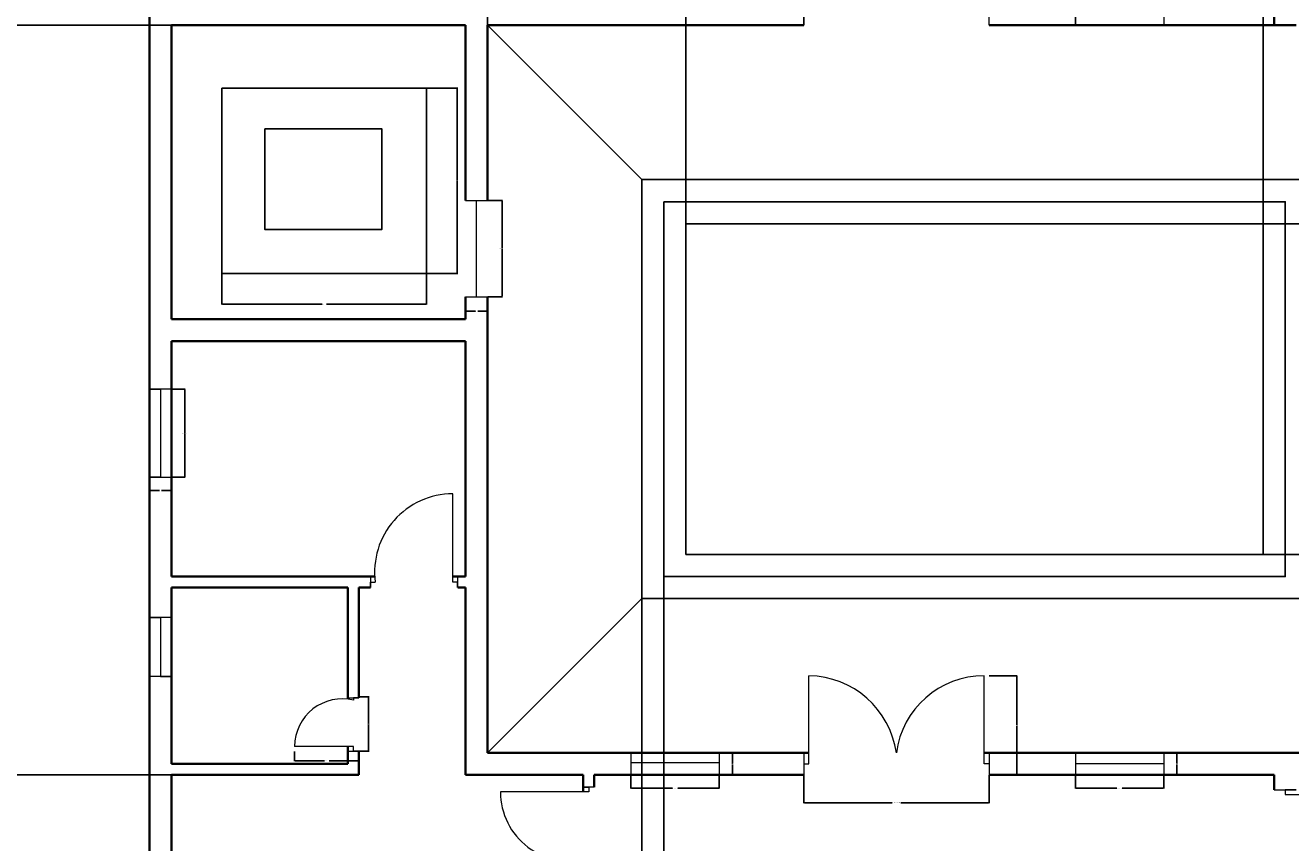
# Model space of a CAD drawing. Units: inches. Extents: x 2185 to 4426, y 1138 to 3073.
# Tile 9 of 14: x 3160 to 3677, y 1501 to 1834. Entities that reach past the tile are written whole.
import ezdxf

# ---------------------------------------------------------------- set-up
doc = ezdxf.new("R2010")
doc.units = ezdxf.units.IN
for name, color, linetype, lineweight in [('A-ANNO-DIMS', 2, 'Continuous', 18), ('A-DOOR', 3, 'Continuous', 18), ('A-FLOR-EDGE', 7, 'Continuous', 25), ('A-GLAZ', 4, 'Continuous', 18), ('A-SITE-WELL', 7, 'Continuous', 25), ('A-WALL', 7, 'Continuous', 35)]:
    doc.layers.add(name, color=color, linetype=linetype, lineweight=lineweight)
doc.styles.get("Standard").update_dxf_attribs({"font": 'arial.ttf'})
doc.dimstyles.get("Standard").update_dxf_attribs({"dimtxt": 0.18, "dimasz": 0.18, "dimexe": 0.18, "dimexo": 0.0625, "dimgap": 0.09, "dimtad": 0, "dimtih": 1, "dimtoh": 1, "dimdec": 4, "dimzin": 0, "dimdsep": 46, "dimtxsty": 'Standard', "dimcen": 0.09, "dimadec": 0, "dimazin": 0, "dimtfac": 1, "dimtdec": 4, "dimtofl": 0, "dimtmove": 0, "dimatfit": 3, "dimfxl": 1, "dimtolj": 1, "dimtzin": 0, "dimarcsym": 0})

# ---------------------------------------------------------------- blocks, each defined once
blk = doc.blocks.new('DOOR-SGL-24-BATH-W')
for p, q in [((21.75, 21.83), (26.25, 21.83)), ((26.25, 21.83), (24, 21.83)), ((24, 21.83), (24, 20.83)), ((24, 2), (0, 2)), ((24, 0), (24, 2)), ((21.75, 0), (26.25, 0)), ((26.25, 0), (24, 0))]:
    blk.add_line(p, q)
blk.add_arc((19.38, 2), 19.38, 76.226, 180)
blk = doc.blocks.new('DOOR-SGL-36-READING')
for p, q in [((33.62, 2.25), (33.62, 38.25)), ((0, 4.5), (0, 0)), ((0, 0), (0, 2.25)), ((0, 2.25), (2, 2.25)), ((35.62, 2.25), (33.62, 2.25)), ((35.62, 4.5), (35.62, 0)), ((35.62, 0), (35.62, 2.25))]:
    blk.add_line(p, q)
blk.add_arc((33.62, 6.36), 31.89, 90, 187.4032)
blk = doc.blocks.new('DOOR-PAIR-36-DINING')
for p, q in [((2, 4.5), (2, 40.5)), ((73.51, 4.5), (73.51, 40.5)), ((0, 9), (0, 0)), ((75.51, 0), (75.51, 9)), ((75.51, 9), (75.51, 4.5)), ((0, 0), (0, 4.5)), ((0, 4.5), (2, 4.5)), ((75.51, 4.5), (73.51, 4.5))]:
    blk.add_line(p, q)
for centre, radius, start, end in [((2, 3.7), 36.8, 8.2761, 90), ((74.14, 4.5), 36.01, 90.9934, 172.8203)]:
    blk.add_arc(centre, radius, start, end)
blk = doc.blocks.new('DOOR-SGL-36-BED-SW')
for p, q in [((38.25, 31.13), (33.75, 31.13)), ((33.75, 31.13), (36, 31.13)), ((36, 31.13), (36, 29.13)), ((36, 29.13), (0, 29.13)), ((36, 0), (36, 2)), ((33.75, 0), (38.25, 0)), ((38.25, 0), (36, 0))]:
    blk.add_line(p, q)
blk.add_arc((28.22, 29.13), 28.22, 180, 285.9925)
blk = doc.blocks.new('DOOR-PAIR-36-VERANDA')
for p, q in [((2, 4.5), (2, 40.5)), ((73.51, 4.5), (73.51, 40.5)), ((0, 9), (0, 0)), ((75.51, 9), (75.51, 0)), ((0, 4.5), (2, 4.5)), ((75.51, 4.5), (73.51, 4.5))]:
    blk.add_line(p, q)
for centre, radius, start, end in [((1.42, 3.87), 36.64, 8.0545, 89.0928), ((73.51, 4.39), 36.11, 90, 172.6635)]:
    blk.add_arc(centre, radius, start, end)
blk = doc.blocks.new('DOOR-SGL-36-BED-S')
for p, q in [((0, 31.73), (9, 31.73)), ((9, 31.73), (4.5, 31.73)), ((4.5, 31.73), (4.5, 31.73)), ((4.5, 31.73), (4.5, 29.73)), ((4.5, 29.73), (40.5, 29.73)), ((0, 0), (9, 0)), ((4.5, 0), (4.5, 2)), ((9, 0), (4.5, 0))]:
    blk.add_line(p, q)
blk.add_arc((11.82, 29.73), 28.68, 255.2109, 0)
blk = doc.blocks.new('WIN-PLAN-24IN-02')
for p, q in [((9, 24), (0, 24)), ((0, 24), (4.5, 24)), ((4.5, 24), (4.5, 0)), ((9, 0), (0, 0)), ((0, 0), (0, 0)), ((4.5, 0), (9, 0))]:
    blk.add_line(p, q)
blk = doc.blocks.new('WIN-PLAN-36IN-01')
for p, q in [((0, 9), (0, 0)), ((36, 4.5), (36, 9)), ((36, 9), (36, 0)), ((0, 0), (0, 4.5)), ((0, 4.5), (0, 4.5)), ((0, 4.5), (36, 4.5))]:
    blk.add_line(p, q)
blk = doc.blocks.new('WIN-PLAN-36IN-03')
for p, q in [((9, 36), (0, 36)), ((0, 36), (0, 36)), ((0, 36), (4.5, 36)), ((4.5, 36), (4.5, 0)), ((4.5, 0), (0, 0)), ((0, 0), (9, 0)), ((9, 0), (9, 0))]:
    blk.add_line(p, q)
blk = doc.blocks.new('WIN-PLAN-36IN-06')
for p, q in [((0, 9), (0, 0)), ((36, 9), (36, 0)), ((0, 5.12), (36, 5.12)), ((36, 5.12), (36, 5.12))]:
    blk.add_line(p, q)
blk = doc.blocks.new('WIN-PLAN-36IN-07')
for p, q in [((0, 9), (0, 0)), ((36, 9), (36, 0)), ((36, 4.5), (0, 4.5))]:
    blk.add_line(p, q)
blk = doc.blocks.new('WIN-PLAN-39IN')
for p, q in [((0, 39.26), (9, 39.26)), ((4.5, 0), (4.5, 39.26)), ((0, 0), (9, 0))]:
    blk.add_line(p, q)
blk = doc.blocks.new('WELL-PLAN')
for points in [[(0, 75.64), (83.5, 75.64), (83.5, 0), (0, 0)], [(17.44, 59), (65.29, 59), (65.29, 18), (17.44, 18)]]:
    blk.add_lwpolyline(points, close=True)
blk = doc.blocks.new('*D72')
at = {"layer": 'A-ANNO-DIMS', "color": 0, "lineweight": -2, "transparency": 16777216}
for p, q in [((3270.1, 1537.99), (3270.1, 1533.94)), ((3270.28, 1534.12), (3282.29, 1534.12)), ((3296.17, 1534.12), (3284.16, 1534.12)), ((3296.35, 1537.99), (3296.35, 1533.94))]:
    blk.add_line(p, q, dxfattribs=at)
at = {"layer": 'A-ANNO-DIMS', "color": 0, "transparency": 16777216}
for points in [[(3270.28, 1534.15), (3270.28, 1534.09), (3270.1, 1534.12)], [(3296.17, 1534.15), (3296.17, 1534.09), (3296.35, 1534.12)]]:
    blk.add_solid(points, dxfattribs=at)
at = {"layer": 'Defpoints', "color": 0, "transparency": 16777216}
for p in [(3270.1, 1538.05), (3296.35, 1538.05), (3296.35, 1534.12)]:
    blk.add_point(p, dxfattribs=at)
at = {"layer": 'A-ANNO-DIMS', "color": 0, "transparency": 16777216, "insert": (3283.22, 1534.12), "char_height": 0.18, "attachment_point": 5}
blk.add_mtext('\\A1;DOOR 26 TYP.', dxfattribs=at)
blk = doc.blocks.new('*D73')
at = {"layer": 'A-ANNO-DIMS', "color": 0, "lineweight": -2, "transparency": 16777216}
for p, q in [((3296.41, 1560.3), (3300.47, 1560.3)), ((3300.29, 1560.12), (3300.29, 1549.36)), ((3300.29, 1538.23), (3300.29, 1549)), ((3296.41, 1538.05), (3300.47, 1538.05))]:
    blk.add_line(p, q, dxfattribs=at)
at = {"layer": 'A-ANNO-DIMS', "color": 0, "transparency": 16777216}
for points in [[(3300.26, 1560.12), (3300.32, 1560.12), (3300.29, 1560.3)], [(3300.26, 1538.23), (3300.32, 1538.23), (3300.29, 1538.05)]]:
    blk.add_solid(points, dxfattribs=at)
at = {"layer": 'Defpoints', "color": 0, "transparency": 16777216}
for p in [(3296.35, 1560.3), (3300.29, 1560.3), (3296.35, 1538.05)]:
    blk.add_point(p, dxfattribs=at)
at = {"layer": 'A-ANNO-DIMS', "color": 0, "transparency": 16777216, "insert": (3300.29, 1549.18), "char_height": 0.18, "attachment_point": 5}
blk.add_mtext('\\A1;22 TYP.', dxfattribs=at)
blk = doc.blocks.new('*D86')
at = {"layer": 'A-ANNO-DIMS', "color": 0, "lineweight": -2, "transparency": 16777216}
for p, q in [((3477.97, 1528.31), (3477.97, 1516.87)), ((3553.49, 1528.31), (3553.49, 1516.87)), ((3478.15, 1517.05), (3513.97, 1517.05)), ((3553.31, 1517.05), (3517.49, 1517.05))]:
    blk.add_line(p, q, dxfattribs=at)
at = {"layer": 'A-ANNO-DIMS', "color": 0, "transparency": 16777216}
for points in [[(3478.15, 1517.08), (3478.15, 1517.02), (3477.97, 1517.05)], [(3553.31, 1517.08), (3553.31, 1517.02), (3553.49, 1517.05)]]:
    blk.add_solid(points, dxfattribs=at)
at = {"layer": 'Defpoints', "color": 0, "transparency": 16777216}
for p in [(3477.97, 1528.38), (3553.49, 1528.38), (3553.49, 1517.05)]:
    blk.add_point(p, dxfattribs=at)
at = {"layer": 'A-ANNO-DIMS', "color": 0, "transparency": 16777216, "insert": (3515.73, 1517.05), "char_height": 0.18, "attachment_point": 5}
blk.add_mtext('\\A1;VERANDAH DOORS 76 TYP.', dxfattribs=at)
blk = doc.blocks.new('*D87')
at = {"layer": 'A-ANNO-DIMS', "color": 0, "lineweight": -2, "transparency": 16777216}
for p, q in [((3553.55, 1568.88), (3564.99, 1568.88)), ((3564.81, 1568.7), (3564.81, 1548.81)), ((3564.81, 1528.56), (3564.81, 1548.45)), ((3553.55, 1528.38), (3564.99, 1528.38))]:
    blk.add_line(p, q, dxfattribs=at)
at = {"layer": 'A-ANNO-DIMS', "color": 0, "transparency": 16777216}
for points in [[(3564.78, 1568.7), (3564.84, 1568.7), (3564.81, 1568.88)], [(3564.78, 1528.56), (3564.84, 1528.56), (3564.81, 1528.38)]]:
    blk.add_solid(points, dxfattribs=at)
at = {"layer": 'Defpoints', "color": 0, "transparency": 16777216}
for p in [(3553.49, 1568.88), (3564.81, 1568.88), (3553.49, 1528.38)]:
    blk.add_point(p, dxfattribs=at)
at = {"layer": 'A-ANNO-DIMS', "color": 0, "transparency": 16777216, "insert": (3564.81, 1548.63), "char_height": 0.18, "attachment_point": 5}
blk.add_mtext('\\A1;41 TYP.', dxfattribs=at)
blk = doc.blocks.new('*D96')
at = {"layer": 'A-ANNO-DIMS', "color": 0, "lineweight": -2, "transparency": 16777216}
for p, q in [((3219.91, 1685.88), (3225.43, 1685.88)), ((3225.25, 1685.7), (3225.25, 1668.07)), ((3225.25, 1650.06), (3225.25, 1667.7)), ((3219.91, 1649.88), (3225.43, 1649.88))]:
    blk.add_line(p, q, dxfattribs=at)
at = {"layer": 'A-ANNO-DIMS', "color": 0, "transparency": 16777216}
for points in [[(3225.22, 1685.7), (3225.28, 1685.7), (3225.25, 1685.88)], [(3225.22, 1650.06), (3225.28, 1650.06), (3225.25, 1649.88)]]:
    blk.add_solid(points, dxfattribs=at)
at = {"layer": 'Defpoints', "color": 0, "transparency": 16777216}
for p in [(3219.85, 1685.88), (3225.25, 1685.88), (3219.85, 1649.88)]:
    blk.add_point(p, dxfattribs=at)
at = {"layer": 'A-ANNO-DIMS', "color": 0, "transparency": 16777216, "insert": (3225.25, 1667.88), "char_height": 0.18, "attachment_point": 5}
blk.add_mtext('\\A1;WINDOW 36 TYP.', dxfattribs=at)
blk = doc.blocks.new('*D97')
at = {"layer": 'A-ANNO-DIMS', "color": 0, "lineweight": -2, "transparency": 16777216}
for p, q in [((3210.85, 1649.82), (3210.85, 1644.3)), ((3219.85, 1649.82), (3219.85, 1644.3)), ((3211.03, 1644.48), (3214.89, 1644.48)), ((3219.67, 1644.48), (3215.81, 1644.48))]:
    blk.add_line(p, q, dxfattribs=at)
at = {"layer": 'A-ANNO-DIMS', "color": 0, "transparency": 16777216}
for points in [[(3211.03, 1644.51), (3211.03, 1644.45), (3210.85, 1644.48)], [(3219.67, 1644.51), (3219.67, 1644.45), (3219.85, 1644.48)]]:
    blk.add_solid(points, dxfattribs=at)
at = {"layer": 'Defpoints', "color": 0, "transparency": 16777216}
for p in [(3210.85, 1649.88), (3219.85, 1649.88), (3219.85, 1644.48)]:
    blk.add_point(p, dxfattribs=at)
at = {"layer": 'A-ANNO-DIMS', "color": 0, "transparency": 16777216, "insert": (3215.35, 1644.48), "char_height": 0.18, "attachment_point": 5}
blk.add_mtext('\\A1;9 TYP.', dxfattribs=at)
blk = doc.blocks.new('*D102')
at = {"layer": 'A-ANNO-DIMS', "color": 0, "lineweight": -2, "transparency": 16777216}
for p, q in [((3407.37, 1528.31), (3407.37, 1522.8)), ((3443.37, 1528.31), (3443.37, 1522.8)), ((3407.55, 1522.98), (3424.25, 1522.98)), ((3443.19, 1522.98), (3426.49, 1522.98))]:
    blk.add_line(p, q, dxfattribs=at)
at = {"layer": 'A-ANNO-DIMS', "color": 0, "transparency": 16777216}
for points in [[(3407.55, 1523.01), (3407.55, 1522.95), (3407.37, 1522.98)], [(3443.19, 1523.01), (3443.19, 1522.95), (3443.37, 1522.98)]]:
    blk.add_solid(points, dxfattribs=at)
at = {"layer": 'Defpoints', "color": 0, "transparency": 16777216}
for p in [(3407.37, 1528.38), (3443.37, 1528.38), (3443.37, 1522.98)]:
    blk.add_point(p, dxfattribs=at)
at = {"layer": 'A-ANNO-DIMS', "color": 0, "transparency": 16777216, "insert": (3425.37, 1522.98), "char_height": 0.18, "attachment_point": 5}
blk.add_mtext('\\A1;WINDOW 36 TYP.', dxfattribs=at)
blk = doc.blocks.new('*D103')
at = {"layer": 'A-ANNO-DIMS', "color": 0, "lineweight": -2, "transparency": 16777216}
for p, q in [((3443.43, 1537.38), (3448.95, 1537.38)), ((3448.77, 1537.2), (3448.77, 1533.06)), ((3448.77, 1528.56), (3448.77, 1532.7)), ((3443.43, 1528.38), (3448.95, 1528.38))]:
    blk.add_line(p, q, dxfattribs=at)
at = {"layer": 'A-ANNO-DIMS', "color": 0, "transparency": 16777216}
for points in [[(3448.74, 1537.2), (3448.8, 1537.2), (3448.77, 1537.38)], [(3448.74, 1528.56), (3448.8, 1528.56), (3448.77, 1528.38)]]:
    blk.add_solid(points, dxfattribs=at)
at = {"layer": 'Defpoints', "color": 0, "transparency": 16777216}
for p in [(3443.37, 1537.38), (3448.77, 1537.38), (3443.37, 1528.38)]:
    blk.add_point(p, dxfattribs=at)
at = {"layer": 'A-ANNO-DIMS', "color": 0, "transparency": 16777216, "insert": (3448.77, 1532.88), "char_height": 0.18, "attachment_point": 5}
blk.add_mtext('\\A1;9 TYP.', dxfattribs=at)
blk = doc.blocks.new('*D104')
at = {"layer": 'A-ANNO-DIMS', "color": 0, "lineweight": -2, "transparency": 16777216}
for p, q in [((3588.76, 1528.31), (3588.76, 1522.8)), ((3624.76, 1528.31), (3624.76, 1522.8)), ((3588.94, 1522.98), (3605.64, 1522.98)), ((3624.58, 1522.98), (3607.88, 1522.98))]:
    blk.add_line(p, q, dxfattribs=at)
at = {"layer": 'A-ANNO-DIMS', "color": 0, "transparency": 16777216}
for points in [[(3588.94, 1523.01), (3588.94, 1522.95), (3588.76, 1522.98)], [(3624.58, 1523.01), (3624.58, 1522.95), (3624.76, 1522.98)]]:
    blk.add_solid(points, dxfattribs=at)
at = {"layer": 'Defpoints', "color": 0, "transparency": 16777216}
for p in [(3588.76, 1528.38), (3624.76, 1528.38), (3624.76, 1522.98)]:
    blk.add_point(p, dxfattribs=at)
at = {"layer": 'A-ANNO-DIMS', "color": 0, "transparency": 16777216, "insert": (3606.76, 1522.98), "char_height": 0.18, "attachment_point": 5}
blk.add_mtext('\\A1;WINDOW 36 TYP.', dxfattribs=at)
blk = doc.blocks.new('*D105')
at = {"layer": 'A-ANNO-DIMS', "color": 0, "lineweight": -2, "transparency": 16777216}
for p, q in [((3624.82, 1537.38), (3630.34, 1537.38)), ((3630.16, 1537.2), (3630.16, 1533.06)), ((3630.16, 1528.56), (3630.16, 1532.7)), ((3624.82, 1528.38), (3630.34, 1528.38))]:
    blk.add_line(p, q, dxfattribs=at)
at = {"layer": 'A-ANNO-DIMS', "color": 0, "transparency": 16777216}
for points in [[(3630.13, 1537.2), (3630.19, 1537.2), (3630.16, 1537.38)], [(3630.13, 1528.56), (3630.19, 1528.56), (3630.16, 1528.38)]]:
    blk.add_solid(points, dxfattribs=at)
at = {"layer": 'Defpoints', "color": 0, "transparency": 16777216}
for p in [(3624.76, 1537.38), (3630.16, 1537.38), (3624.76, 1528.38)]:
    blk.add_point(p, dxfattribs=at)
at = {"layer": 'A-ANNO-DIMS', "color": 0, "transparency": 16777216, "insert": (3630.16, 1532.88), "char_height": 0.18, "attachment_point": 5}
blk.add_mtext('\\A1;9 TYP.', dxfattribs=at)
blk = doc.blocks.new('*D112')
at = {"layer": 'A-ANNO-DIMS', "color": 0, "lineweight": -2, "transparency": 16777216}
for p, q in [((3348.91, 1762.84), (3354.92, 1762.84)), ((3354.74, 1762.66), (3354.74, 1743.4)), ((3354.74, 1723.77), (3354.74, 1743.03)), ((3348.91, 1723.59), (3354.92, 1723.59))]:
    blk.add_line(p, q, dxfattribs=at)
at = {"layer": 'A-ANNO-DIMS', "color": 0, "transparency": 16777216}
for points in [[(3354.71, 1762.66), (3354.77, 1762.66), (3354.74, 1762.84)], [(3354.71, 1723.77), (3354.77, 1723.77), (3354.74, 1723.59)]]:
    blk.add_solid(points, dxfattribs=at)
at = {"layer": 'Defpoints', "color": 0, "transparency": 16777216}
for p in [(3348.85, 1762.84), (3354.74, 1762.84), (3348.85, 1723.59)]:
    blk.add_point(p, dxfattribs=at)
at = {"layer": 'A-ANNO-DIMS', "color": 0, "transparency": 16777216, "insert": (3354.74, 1743.21), "char_height": 0.18, "attachment_point": 5}
blk.add_mtext('\\A1;WINDOW 39 TYP.', dxfattribs=at)
blk = doc.blocks.new('*D113')
at = {"layer": 'A-ANNO-DIMS', "color": 0, "lineweight": -2, "transparency": 16777216}
for p, q in [((3339.85, 1723.52), (3339.85, 1717.52)), ((3348.85, 1723.52), (3348.85, 1717.52)), ((3340.03, 1717.7), (3343.89, 1717.7)), ((3348.67, 1717.7), (3344.81, 1717.7))]:
    blk.add_line(p, q, dxfattribs=at)
at = {"layer": 'A-ANNO-DIMS', "color": 0, "transparency": 16777216}
for points in [[(3340.03, 1717.73), (3340.03, 1717.67), (3339.85, 1717.7)], [(3348.67, 1717.73), (3348.67, 1717.67), (3348.85, 1717.7)]]:
    blk.add_solid(points, dxfattribs=at)
at = {"layer": 'Defpoints', "color": 0, "transparency": 16777216}
for p in [(3339.85, 1723.59), (3348.85, 1723.59), (3348.85, 1717.7)]:
    blk.add_point(p, dxfattribs=at)
at = {"layer": 'A-ANNO-DIMS', "color": 0, "transparency": 16777216, "insert": (3344.35, 1717.7), "char_height": 0.18, "attachment_point": 5}
blk.add_mtext('\\A1;9 TYP.', dxfattribs=at)
blk = doc.blocks.new('*D118')
at = {"layer": 'A-ANNO-DIMS', "color": 0, "lineweight": -2, "transparency": 16777216}
for p, q in [((3240.45, 1733), (3240.45, 1720.36)), ((3323.95, 1733), (3323.95, 1720.36)), ((3240.63, 1720.54), (3281.29, 1720.54)), ((3323.77, 1720.54), (3283.11, 1720.54))]:
    blk.add_line(p, q, dxfattribs=at)
at = {"layer": 'A-ANNO-DIMS', "color": 0, "transparency": 16777216}
for points in [[(3240.63, 1720.57), (3240.63, 1720.51), (3240.45, 1720.54)], [(3323.77, 1720.57), (3323.77, 1720.51), (3323.95, 1720.54)]]:
    blk.add_solid(points, dxfattribs=at)
at = {"layer": 'Defpoints', "color": 0, "transparency": 16777216}
for p in [(3240.45, 1733.06), (3323.95, 1733.06), (3323.95, 1720.54)]:
    blk.add_point(p, dxfattribs=at)
at = {"layer": 'A-ANNO-DIMS', "color": 0, "transparency": 16777216, "insert": (3282.2, 1720.54), "char_height": 0.18, "attachment_point": 5}
blk.add_mtext('\\A1;WELL 84 TYP.', dxfattribs=at)
blk = doc.blocks.new('*D119')
at = {"layer": 'A-ANNO-DIMS', "color": 0, "lineweight": -2, "transparency": 16777216}
for p, q in [((3324.01, 1808.7), (3336.66, 1808.7)), ((3336.48, 1808.52), (3336.48, 1771.06)), ((3336.48, 1733.24), (3336.48, 1770.7)), ((3324.01, 1733.06), (3336.66, 1733.06))]:
    blk.add_line(p, q, dxfattribs=at)
at = {"layer": 'A-ANNO-DIMS', "color": 0, "transparency": 16777216}
for points in [[(3336.45, 1808.52), (3336.51, 1808.52), (3336.48, 1808.7)], [(3336.45, 1733.24), (3336.51, 1733.24), (3336.48, 1733.06)]]:
    blk.add_solid(points, dxfattribs=at)
at = {"layer": 'Defpoints', "color": 0, "transparency": 16777216}
for p in [(3323.95, 1808.7), (3336.48, 1808.7), (3323.95, 1733.06)]:
    blk.add_point(p, dxfattribs=at)
at = {"layer": 'A-ANNO-DIMS', "color": 0, "transparency": 16777216, "insert": (3336.48, 1770.88), "char_height": 0.18, "attachment_point": 5}
blk.add_mtext('\\A1;76 TYP.', dxfattribs=at)
blk = doc.blocks.new('*D150')
at = {"layer": 'A-ANNO-DIMS', "color": 0, "lineweight": -2, "transparency": 16777216}
for p, q in [((3219.79, 1528.38), (3101.64, 1528.38)), ((3101.82, 1528.2), (3101.82, 1428.06)), ((3101.82, 1327.56), (3101.82, 1427.7)), ((3210.79, 1327.38), (3101.64, 1327.38))]:
    blk.add_line(p, q, dxfattribs=at)
at = {"layer": 'A-ANNO-DIMS', "color": 0, "transparency": 16777216}
for points in [[(3101.79, 1528.2), (3101.85, 1528.2), (3101.82, 1528.38)], [(3101.79, 1327.56), (3101.85, 1327.56), (3101.82, 1327.38)]]:
    blk.add_solid(points, dxfattribs=at)
at = {"layer": 'Defpoints', "color": 0, "transparency": 16777216}
for p in [(3101.82, 1528.38), (3219.85, 1528.38), (3210.85, 1327.38)]:
    blk.add_point(p, dxfattribs=at)
at = {"layer": 'A-ANNO-DIMS', "color": 0, "transparency": 16777216, "insert": (3101.82, 1427.88), "char_height": 0.18, "attachment_point": 5}
blk.add_mtext('\\A1;201', dxfattribs=at)
blk = doc.blocks.new('*D151')
at = {"layer": 'A-ANNO-DIMS', "color": 0, "lineweight": -2, "transparency": 16777216}
for p, q in [((3219.79, 1834.38), (3101.64, 1834.38)), ((3101.82, 1834.2), (3101.82, 1681.56)), ((3101.82, 1528.56), (3101.82, 1681.19)), ((3219.79, 1528.38), (3101.64, 1528.38))]:
    blk.add_line(p, q, dxfattribs=at)
at = {"layer": 'A-ANNO-DIMS', "color": 0, "transparency": 16777216}
for points in [[(3101.79, 1834.2), (3101.85, 1834.2), (3101.82, 1834.38)], [(3101.79, 1528.56), (3101.85, 1528.56), (3101.82, 1528.38)]]:
    blk.add_solid(points, dxfattribs=at)
at = {"layer": 'Defpoints', "color": 0, "transparency": 16777216}
for p in [(3101.82, 1834.38), (3219.85, 1834.38), (3219.85, 1528.38)]:
    blk.add_point(p, dxfattribs=at)
at = {"layer": 'A-ANNO-DIMS', "color": 0, "transparency": 16777216, "insert": (3101.82, 1681.38), "char_height": 0.18, "attachment_point": 5}
blk.add_mtext('\\A1;306', dxfattribs=at)
blk = doc.blocks.new('*D152')
at = {"layer": 'A-ANNO-DIMS', "color": 0, "lineweight": -2, "transparency": 16777216}
for p, q in [((3155.01, 1880.56), (3101.64, 1880.56)), ((3101.82, 1880.38), (3101.82, 1857.65)), ((3101.82, 1834.56), (3101.82, 1857.29)), ((3219.79, 1834.38), (3101.64, 1834.38))]:
    blk.add_line(p, q, dxfattribs=at)
at = {"layer": 'A-ANNO-DIMS', "color": 0, "transparency": 16777216}
for points in [[(3101.79, 1880.38), (3101.85, 1880.38), (3101.82, 1880.56)], [(3101.79, 1834.56), (3101.85, 1834.56), (3101.82, 1834.38)]]:
    blk.add_solid(points, dxfattribs=at)
at = {"layer": 'Defpoints', "color": 0, "transparency": 16777216}
for p in [(3101.82, 1880.56), (3155.07, 1880.56), (3219.85, 1834.38)]:
    blk.add_point(p, dxfattribs=at)
at = {"layer": 'A-ANNO-DIMS', "color": 0, "transparency": 16777216, "insert": (3101.82, 1857.47), "char_height": 0.18, "attachment_point": 5}
blk.add_mtext('\\A1;46.19', dxfattribs=at)
blk = doc.blocks.new('*D155')
at = {"layer": 'A-ANNO-DIMS', "color": 0, "lineweight": -2, "transparency": 16777216}
for p, q in [((3348.85, 1834.44), (3348.85, 2379.81)), ((3349.03, 2379.63), (3388.93, 2379.63)), ((3429.63, 2379.63), (3389.72, 2379.63)), ((3429.81, 1753.44), (3429.81, 2379.81))]:
    blk.add_line(p, q, dxfattribs=at)
at = {"layer": 'A-ANNO-DIMS', "color": 0, "transparency": 16777216}
for points in [[(3349.03, 2379.66), (3349.03, 2379.6), (3348.85, 2379.63)], [(3429.63, 2379.66), (3429.63, 2379.6), (3429.81, 2379.63)]]:
    blk.add_solid(points, dxfattribs=at)
at = {"layer": 'Defpoints', "color": 0, "transparency": 16777216}
for p in [(3429.81, 2379.63), (3348.85, 1834.38), (3429.81, 1753.38)]:
    blk.add_point(p, dxfattribs=at)
at = {"layer": 'A-ANNO-DIMS', "color": 0, "transparency": 16777216, "insert": (3389.33, 2379.63), "char_height": 0.18, "attachment_point": 5}
blk.add_mtext('\\A1;80.96', dxfattribs=at)
blk = doc.blocks.new('*D156')
at = {"layer": 'A-ANNO-DIMS', "color": 0, "lineweight": -2, "transparency": 16777216}
for p, q in [((3429.81, 1753.44), (3429.81, 2379.81)), ((3429.99, 2379.63), (3547.11, 2379.63)), ((3665.17, 2379.63), (3548.04, 2379.63)), ((3665.35, 1753.44), (3665.35, 2379.81))]:
    blk.add_line(p, q, dxfattribs=at)
at = {"layer": 'A-ANNO-DIMS', "color": 0, "transparency": 16777216}
for points in [[(3429.99, 2379.66), (3429.99, 2379.6), (3429.81, 2379.63)], [(3665.17, 2379.66), (3665.17, 2379.6), (3665.35, 2379.63)]]:
    blk.add_solid(points, dxfattribs=at)
at = {"layer": 'Defpoints', "color": 0, "transparency": 16777216}
for p in [(3665.35, 2379.63), (3429.81, 1753.38), (3665.35, 1753.38)]:
    blk.add_point(p, dxfattribs=at)
at = {"layer": 'A-ANNO-DIMS', "color": 0, "transparency": 16777216, "insert": (3547.58, 2379.63), "char_height": 0.18, "attachment_point": 5}
blk.add_mtext('\\A1;235.54', dxfattribs=at)
blk = doc.blocks.new('*D157')
at = {"layer": 'A-ANNO-DIMS', "color": 0, "lineweight": -2, "transparency": 16777216}
for p, q in [((3665.35, 1753.44), (3665.35, 2379.81)), ((3665.53, 2379.63), (3705.65, 2379.63)), ((3746.17, 2379.63), (3706.05, 2379.63)), ((3746.35, 1834.44), (3746.35, 2379.81))]:
    blk.add_line(p, q, dxfattribs=at)
at = {"layer": 'A-ANNO-DIMS', "color": 0, "transparency": 16777216}
for points in [[(3665.53, 2379.66), (3665.53, 2379.6), (3665.35, 2379.63)], [(3746.17, 2379.66), (3746.17, 2379.6), (3746.35, 2379.63)]]:
    blk.add_solid(points, dxfattribs=at)
at = {"layer": 'Defpoints', "color": 0, "transparency": 16777216}
for p in [(3746.35, 2379.63), (3746.35, 1834.38), (3665.35, 1753.38)]:
    blk.add_point(p, dxfattribs=at)
at = {"layer": 'A-ANNO-DIMS', "color": 0, "transparency": 16777216, "insert": (3705.85, 2379.63), "char_height": 0.18, "attachment_point": 5}
blk.add_mtext('\\A1;81', dxfattribs=at)
blk = doc.blocks.new('*D158')
at = {"layer": 'A-ANNO-DIMS', "color": 0, "lineweight": -2, "transparency": 16777216}
for p, q in [((3665.41, 1618.38), (4058.64, 1618.38)), ((4058.46, 1618.2), (4058.46, 1578.06)), ((4058.46, 1537.56), (4058.46, 1577.7)), ((3746.41, 1537.38), (4058.64, 1537.38))]:
    blk.add_line(p, q, dxfattribs=at)
at = {"layer": 'A-ANNO-DIMS', "color": 0, "transparency": 16777216}
for points in [[(4058.43, 1618.2), (4058.49, 1618.2), (4058.46, 1618.38)], [(4058.43, 1537.56), (4058.49, 1537.56), (4058.46, 1537.38)]]:
    blk.add_solid(points, dxfattribs=at)
at = {"layer": 'Defpoints', "color": 0, "transparency": 16777216}
for p in [(3665.35, 1618.38), (4058.46, 1618.38), (3746.35, 1537.38)]:
    blk.add_point(p, dxfattribs=at)
at = {"layer": 'A-ANNO-DIMS', "color": 0, "transparency": 16777216, "insert": (4058.46, 1577.88), "char_height": 0.18, "attachment_point": 5}
blk.add_mtext('\\A1;81', dxfattribs=at)
blk = doc.blocks.new('*D159')
at = {"layer": 'A-ANNO-DIMS', "color": 0, "lineweight": -2, "transparency": 16777216}
for p, q in [((3665.41, 1753.38), (4058.64, 1753.38)), ((4058.46, 1753.2), (4058.46, 1686.06)), ((4058.46, 1618.56), (4058.46, 1685.69)), ((3665.41, 1618.38), (4058.64, 1618.38))]:
    blk.add_line(p, q, dxfattribs=at)
at = {"layer": 'A-ANNO-DIMS', "color": 0, "transparency": 16777216}
for points in [[(4058.43, 1753.2), (4058.49, 1753.2), (4058.46, 1753.38)], [(4058.43, 1618.56), (4058.49, 1618.56), (4058.46, 1618.38)]]:
    blk.add_solid(points, dxfattribs=at)
at = {"layer": 'Defpoints', "color": 0, "transparency": 16777216}
for p in [(3665.35, 1753.38), (4058.46, 1753.38), (3665.35, 1618.38)]:
    blk.add_point(p, dxfattribs=at)
at = {"layer": 'A-ANNO-DIMS', "color": 0, "transparency": 16777216, "insert": (4058.46, 1685.88), "char_height": 0.18, "attachment_point": 5}
blk.add_mtext('\\A1;135', dxfattribs=at)
blk = doc.blocks.new('*D160')
at = {"layer": 'A-ANNO-DIMS', "color": 0, "lineweight": -2, "transparency": 16777216}
for p, q in [((3746.41, 1834.38), (4058.64, 1834.38)), ((4058.46, 1834.2), (4058.46, 1794.06)), ((4058.46, 1753.56), (4058.46, 1793.7)), ((3665.41, 1753.38), (4058.64, 1753.38))]:
    blk.add_line(p, q, dxfattribs=at)
at = {"layer": 'A-ANNO-DIMS', "color": 0, "transparency": 16777216}
for points in [[(4058.43, 1834.2), (4058.49, 1834.2), (4058.46, 1834.38)], [(4058.43, 1753.56), (4058.49, 1753.56), (4058.46, 1753.38)]]:
    blk.add_solid(points, dxfattribs=at)
at = {"layer": 'Defpoints', "color": 0, "transparency": 16777216}
for p in [(3746.35, 1834.38), (4058.46, 1834.38), (3665.35, 1753.38)]:
    blk.add_point(p, dxfattribs=at)
at = {"layer": 'A-ANNO-DIMS', "color": 0, "transparency": 16777216, "insert": (4058.46, 1793.88), "char_height": 0.18, "attachment_point": 5}
blk.add_mtext('\\A1;81', dxfattribs=at)
blk = doc.blocks.new('*D161')
at = {"layer": 'A-ANNO-DIMS', "color": 0, "lineweight": -2, "transparency": 16777216}
for p, q in [((3420.81, 1609.31), (3420.81, 1273.95)), ((3411.81, 1600.31), (3411.81, 1273.95)), ((3411.99, 1274.13), (3416.16, 1274.13)), ((3420.63, 1274.13), (3416.46, 1274.13))]:
    blk.add_line(p, q, dxfattribs=at)
at = {"layer": 'A-ANNO-DIMS', "color": 0, "transparency": 16777216}
for points in [[(3411.99, 1274.16), (3411.99, 1274.1), (3411.81, 1274.13)], [(3420.63, 1274.16), (3420.63, 1274.1), (3420.81, 1274.13)]]:
    blk.add_solid(points, dxfattribs=at)
at = {"layer": 'Defpoints', "color": 0, "transparency": 16777216}
for p in [(3420.81, 1609.38), (3411.81, 1600.38), (3420.81, 1274.13)]:
    blk.add_point(p, dxfattribs=at)
at = {"layer": 'A-ANNO-DIMS', "color": 0, "transparency": 16777216, "insert": (3416.31, 1274.13), "char_height": 0.18, "attachment_point": 5}
blk.add_mtext('\\A1;9', dxfattribs=at)

msp = doc.modelspace()

# ---------------------------------------------------------------- linework, layer by layer
at = {"layer": 'A-FLOR-EDGE'}
for p, q in [((3411.807, 1771.377), (3348.849, 1834.377)), ((3411.807, 1771.377), (3348.849, 1834.377)), ((3674.349, 1762.377), (3420.807, 1762.377)), ((3420.807, 1762.377), (3420.807, 1609.377)), ((3674.349, 1762.377), (3420.807, 1762.377)), ((3420.807, 1762.377), (3420.807, 1609.377)), ((3674.349, 1609.377), (3674.349, 1762.377)), ((3674.349, 1609.377), (3674.349, 1762.377)), ((3420.807, 1609.377), (3674.349, 1609.377)), ((3420.807, 1609.377), (3674.349, 1609.377)), ((3411.807, 1600.377), (3348.849, 1537.377)), ((3411.807, 1600.377), (3348.849, 1537.377))]:
    msp.add_line(p, q, dxfattribs=at)
for points in [[(3411.807, 1771.377), (3683.349, 1771.377), (3683.349, 1600.377), (3411.807, 1600.377)], [(3411.807, 1771.377), (3683.349, 1771.377), (3683.349, 1600.377), (3411.807, 1600.377)], [(3420.807, 1762.377), (3674.349, 1762.377), (3674.349, 1609.377), (3420.807, 1609.377)], [(3420.807, 1762.377), (3674.349, 1762.377), (3674.349, 1609.377), (3420.807, 1609.377)], [(3429.807, 1753.377), (3665.349, 1753.377), (3665.349, 1618.377), (3429.807, 1618.377)], [(3429.807, 1753.377), (3665.349, 1753.377), (3665.349, 1618.377), (3429.807, 1618.377)]]:
    msp.add_lwpolyline(points, close=True, dxfattribs=at)
at = {"layer": 'A-WALL'}
for p, q in [((3210.849, 2136.303), (3210.849, 1327.377)), ((3210.849, 2136.303), (3210.849, 1327.377)), ((3210.849, 2136.303), (3210.849, 1327.377)), ((3210.849, 2136.303), (3210.849, 1327.377)), ((3669.849, 1843.377), (3669.849, 1834.377)), ((3669.849, 1843.377), (3669.849, 1834.377)), ((3219.849, 1834.377), (3219.849, 1714.377)), ((3219.849, 1834.377), (3339.849, 1834.377)), ((3219.849, 1834.377), (3219.849, 1714.377)), ((3219.849, 1834.377), (3339.849, 1834.377)), ((3339.849, 1834.377), (3339.849, 1762.843)), ((3339.849, 1834.377), (3339.849, 1762.843)), ((3348.849, 1834.377), (3348.849, 1762.843)), ((3348.849, 1834.377), (3363.849, 1834.377)), ((3348.849, 1834.377), (3348.849, 1762.843)), ((3348.849, 1834.377), (3363.849, 1834.377)), ((3363.849, 1834.377), (3477.974, 1834.377)), ((3363.849, 1834.377), (3477.974, 1834.377)), ((3553.486, 1834.377), (3678.849, 1834.377)), ((3553.486, 1834.377), (3678.849, 1834.377)), ((3339.849, 1723.587), (3339.849, 1714.377)), ((3339.849, 1723.587), (3339.849, 1714.377)), ((3348.849, 1723.587), (3348.849, 1705.377)), ((3348.849, 1723.587), (3348.849, 1705.377)), ((3219.849, 1714.377), (3339.849, 1714.377)), ((3219.849, 1714.377), (3339.849, 1714.377)), ((3219.849, 1705.377), (3219.849, 1609.377)), ((3219.849, 1705.377), (3339.849, 1705.377)), ((3219.849, 1705.377), (3219.849, 1609.377)), ((3219.849, 1705.377), (3219.849, 1609.377)), ((3219.849, 1705.377), (3339.849, 1705.377)), ((3219.849, 1705.377), (3219.849, 1609.377)), ((3339.849, 1609.377), (3339.849, 1705.377)), ((3339.849, 1609.377), (3339.849, 1705.377)), ((3348.849, 1705.377), (3348.849, 1537.377)), ((3348.849, 1705.377), (3348.849, 1537.377)), ((3219.849, 1609.377), (3302.8, 1609.377)), ((3219.849, 1609.377), (3302.8, 1609.377)), ((3334.636, 1609.377), (3339.849, 1609.377)), ((3334.636, 1609.377), (3339.849, 1609.377)), ((3348.849, 1609.377), (3348.849, 1604.877)), ((3348.849, 1537.377), (3348.849, 1609.377)), ((3348.849, 1609.377), (3348.849, 1604.877)), ((3348.849, 1537.377), (3348.849, 1609.377)), ((3219.849, 1604.877), (3219.849, 1532.877)), ((3291.849, 1604.877), (3219.849, 1604.877)), ((3219.849, 1604.877), (3219.849, 1532.877)), ((3219.849, 1604.877), (3219.849, 1532.877)), ((3291.849, 1604.877), (3219.849, 1604.877)), ((3219.849, 1604.877), (3219.849, 1532.877)), ((3291.849, 1559.295), (3291.849, 1604.877)), ((3291.849, 1559.295), (3291.849, 1604.877)), ((3301.011, 1604.877), (3296.349, 1604.877)), ((3296.349, 1604.877), (3296.349, 1559.882)), ((3301.011, 1604.877), (3296.349, 1604.877)), ((3296.349, 1604.877), (3296.349, 1559.882)), ((3339.849, 1604.877), (3336.636, 1604.877)), ((3339.849, 1604.877), (3336.636, 1604.877)), ((3339.849, 1537.377), (3339.849, 1604.877)), ((3339.849, 1537.377), (3339.849, 1604.877)), ((3291.849, 1532.877), (3291.849, 1540.055)), ((3291.849, 1532.877), (3291.849, 1540.055)), ((3296.349, 1538.055), (3296.349, 1537.377)), ((3296.349, 1538.055), (3296.349, 1537.377)), ((3296.349, 1537.377), (3296.349, 1528.377)), ((3296.349, 1537.377), (3296.349, 1528.377)), ((3339.849, 1537.377), (3339.849, 1528.377)), ((3339.849, 1537.377), (3339.849, 1528.377)), ((3479.974, 1537.377), (3348.849, 1537.377)), ((3348.849, 1537.377), (3348.849, 1537.377)), ((3479.974, 1537.377), (3348.849, 1537.377)), ((3348.849, 1537.377), (3348.849, 1537.377)), ((3588.761, 1537.377), (3551.486, 1537.377)), ((3588.761, 1537.377), (3551.486, 1537.377)), ((3746.349, 1537.377), (3588.761, 1537.377)), ((3746.349, 1537.377), (3588.761, 1537.377)), ((3219.849, 1532.877), (3291.849, 1532.877)), ((3219.849, 1532.877), (3291.849, 1532.877)), ((3219.849, 1532.877), (3291.849, 1532.877)), ((3219.849, 1532.877), (3291.849, 1532.877)), ((3267.849, 1532.877), (3291.849, 1532.877)), ((3267.849, 1532.877), (3291.849, 1532.877)), ((3219.849, 1528.377), (3219.849, 1336.377)), ((3296.349, 1528.377), (3219.849, 1528.377)), ((3219.849, 1528.377), (3219.849, 1336.377)), ((3219.849, 1528.377), (3219.849, 1336.377)), ((3296.349, 1528.377), (3219.849, 1528.377)), ((3219.849, 1528.377), (3219.849, 1336.377)), ((3296.349, 1528.377), (3296.349, 1528.377)), ((3296.349, 1528.377), (3296.349, 1528.377)), ((3387.849, 1528.377), (3339.849, 1528.377)), ((3387.849, 1528.377), (3339.849, 1528.377)), ((3387.849, 1521.439), (3387.849, 1528.377)), ((3387.849, 1521.439), (3387.849, 1528.377)), ((3477.974, 1528.377), (3392.349, 1528.377)), ((3392.349, 1528.377), (3392.349, 1523.439)), ((3477.974, 1528.377), (3392.349, 1528.377)), ((3392.349, 1528.377), (3392.349, 1523.439)), ((3588.761, 1528.377), (3553.486, 1528.377)), ((3588.761, 1528.377), (3553.486, 1528.377)), ((3669.849, 1528.377), (3588.761, 1528.377)), ((3669.849, 1528.377), (3588.761, 1528.377)), ((3669.849, 1528.377), (3669.849, 1522.356)), ((3669.849, 1528.377), (3669.849, 1522.356))]:
    msp.add_line(p, q, dxfattribs=at)

# ---------------------------------------------------------------- block references
at = {"layer": 'A-DOOR'}
for name, p in [('DOOR-PAIR-36-DINING', (3477.974, 1834.377)), ('DOOR-PAIR-36-DINING', (3477.974, 1834.377)), ('DOOR-SGL-36-READING', (3301.012, 1604.877)), ('DOOR-SGL-36-READING', (3301.012, 1604.877)), ('DOOR-PAIR-36-VERANDA', (3477.974, 1528.377)), ('DOOR-PAIR-36-VERANDA', (3477.974, 1528.377)), ('DOOR-SGL-24-BATH-W', (3270.099, 1538.055)), ('DOOR-SGL-24-BATH-W', (3270.099, 1538.055)), ('DOOR-SGL-36-BED-SW', (3354.099, 1492.307)), ('DOOR-SGL-36-BED-SW', (3354.099, 1492.307)), ('DOOR-SGL-36-BED-S', (3669.849, 1490.627)), ('DOOR-SGL-36-BED-S', (3669.849, 1490.627))]:
    msp.add_blockref(name, p, dxfattribs=at)
at = {"layer": 'A-GLAZ'}
for name, p in [('WIN-PLAN-36IN-01', (3588.761, 1834.377)), ('WIN-PLAN-36IN-01', (3588.761, 1834.377)), ('WIN-PLAN-39IN', (3339.849, 1723.587)), ('WIN-PLAN-39IN', (3339.849, 1723.587)), ('WIN-PLAN-36IN-03', (3210.849, 1649.883)), ('WIN-PLAN-36IN-03', (3210.849, 1649.883)), ('WIN-PLAN-24IN-02', (3210.849, 1568.585)), ('WIN-PLAN-24IN-02', (3210.849, 1568.585)), ('WIN-PLAN-36IN-06', (3407.369, 1528.377)), ('WIN-PLAN-36IN-06', (3407.369, 1528.377)), ('WIN-PLAN-36IN-07', (3588.761, 1528.377)), ('WIN-PLAN-36IN-07', (3588.761, 1528.377))]:
    msp.add_blockref(name, p, dxfattribs=at)
at = {"layer": 'A-SITE-WELL'}
msp.add_blockref('WELL-PLAN', (3240.449, 1733.064), dxfattribs=at)
msp.add_blockref('WELL-PLAN', (3240.449, 1733.064), dxfattribs=at)

# ---------------------------------------------------------------- dimensions: what is measured, and where the dimension line sits
at = {"layer": 'A-ANNO-DIMS'}
for base, p1, p2, override, picture, middle in [((3429.807, 2379.627), (3348.849, 1834.377), (3429.807, 1753.377), {"dimdec": 2, "dimlfac": 1, "dimrnd": 0, "dimzin": 0, "dimdsep": 46, "dimlunit": 2}, '*D155', (3389.328, 2379.627)), ((3665.349, 2379.627), (3429.807, 1753.377), (3665.349, 1753.377), {"dimdec": 2, "dimlfac": 1, "dimrnd": 0, "dimzin": 0, "dimdsep": 46, "dimlunit": 2}, '*D156', (3547.578, 2379.627)), ((3746.349, 2379.627), (3665.349, 1753.377), (3746.349, 1834.377), {"dimdec": 0, "dimlfac": 1, "dimrnd": 0, "dimzin": 0, "dimdsep": 46, "dimlunit": 2}, '*D157', (3705.849, 2379.627)), ((3420.807, 1274.127), (3411.807, 1600.377), (3420.807, 1609.377), {"dimdec": 0, "dimlfac": 1, "dimrnd": 0, "dimzin": 0, "dimdsep": 46, "dimlunit": 2}, '*D161', (3416.307, 1274.127))]:
    dim = msp.add_linear_dim(base=base, p1=p1, p2=p2, dimstyle='Standard', override=override, dxfattribs=at)
    dim.commit()
    dim.dimension.update_dxf_attribs({"geometry": picture, "text_midpoint": middle})
for base, p1, p2, override, picture, middle in [((3101.824, 1880.563), (3219.849, 1834.377), (3155.074, 1880.563), {"dimdec": 2, "dimlfac": 1, "dimrnd": 0, "dimzin": 0, "dimdsep": 46, "dimlunit": 2}, '*D152', (3101.824, 1857.47)), ((3101.824, 1834.377), (3219.849, 1528.377), (3219.849, 1834.377), {"dimdec": 0, "dimlfac": 1, "dimrnd": 0, "dimzin": 0, "dimdsep": 46, "dimlunit": 2}, '*D151', (3101.824, 1681.377)), ((4058.46, 1834.377), (3665.349, 1753.377), (3746.349, 1834.377), {"dimdec": 0, "dimlfac": 1, "dimrnd": 0, "dimzin": 0, "dimdsep": 46, "dimlunit": 2}, '*D160', (4058.46, 1793.877)), ((4058.46, 1753.377), (3665.349, 1618.377), (3665.349, 1753.377), {"dimdec": 0, "dimlfac": 1, "dimrnd": 0, "dimzin": 0, "dimdsep": 46, "dimlunit": 2}, '*D159', (4058.46, 1685.877)), ((4058.46, 1618.377), (3746.349, 1537.377), (3665.349, 1618.377), {"dimdec": 0, "dimlfac": 1, "dimrnd": 0, "dimzin": 0, "dimdsep": 46, "dimlunit": 2}, '*D158', (4058.46, 1577.877)), ((3101.824, 1528.377), (3210.849, 1327.377), (3219.849, 1528.377), {"dimdec": 0, "dimlfac": 1, "dimrnd": 0, "dimzin": 0, "dimdsep": 46, "dimlunit": 2}, '*D150', (3101.824, 1427.877))]:
    dim = msp.add_linear_dim(base=base, p1=p1, p2=p2, angle=90, dimstyle='Standard', override=override, dxfattribs=at)
    dim.commit()
    dim.dimension.update_dxf_attribs({"geometry": picture, "text_midpoint": middle})
for base, p1, p2, text, picture, middle in [((3336.477, 1808.7), (3323.952, 1733.064), (3323.952, 1808.7), '<> TYP.', '*D119', (3336.477, 1770.882)), ((3354.738, 1762.843), (3348.849, 1723.587), (3348.849, 1762.843), 'WINDOW <> TYP.', '*D112', (3354.738, 1743.215)), ((3225.249, 1685.883), (3219.849, 1649.883), (3219.849, 1685.883), 'WINDOW <> TYP.', '*D96', (3225.249, 1667.883)), ((3564.81313659, 1568.876947079), (3553.48629281, 1528.376947079), (3553.48629281, 1568.876947079), '<> TYP.', '*D87', (3564.81313659, 1548.626947079)), ((3300.287, 1560.3), (3296.349, 1538.055), (3296.349, 1560.3), '<> TYP.', '*D73', (3300.287, 1549.177)), ((3448.769, 1537.377), (3443.369, 1528.377), (3443.369, 1537.377), '<> TYP.', '*D103', (3448.769, 1532.877)), ((3630.161, 1537.377), (3624.761, 1528.377), (3624.761, 1537.377), '<> TYP.', '*D105', (3630.161, 1532.877))]:
    dim = msp.add_linear_dim(base=base, p1=p1, p2=p2, angle=90, text=text, dimstyle='Standard', override={"dimdec": 0, "dimlfac": 1, "dimrnd": 0, "dimzin": 0, "dimdsep": 46, "dimlunit": 2}, dxfattribs=at)
    dim.commit()
    dim.dimension.update_dxf_attribs({"geometry": picture, "text_midpoint": middle})
for base, p1, p2, text, picture, middle in [((3323.952, 1720.539), (3240.449, 1733.064), (3323.952, 1733.064), 'WELL <> TYP.', '*D118', (3282.2, 1720.539)), ((3348.849, 1717.698), (3339.849, 1723.587), (3348.849, 1723.587), '<> TYP.', '*D113', (3344.349, 1717.698)), ((3219.849, 1644.483), (3210.849, 1649.883), (3219.849, 1649.883), '<> TYP.', '*D97', (3215.349, 1644.483)), ((3296.349, 1534.117), (3270.099, 1538.055), (3296.349, 1538.055), 'DOOR <> TYP.', '*D72', (3283.224, 1534.117)), ((3443.369, 1522.977), (3407.369, 1528.377), (3443.369, 1528.377), 'WINDOW <> TYP.', '*D102', (3425.369, 1522.977)), ((3553.486, 1517.05), (3477.974, 1528.377), (3553.486, 1528.377), 'VERANDAH DOORS <> TYP.', '*D86', (3515.73, 1517.05)), ((3624.761, 1522.977), (3588.761, 1528.377), (3624.761, 1528.377), 'WINDOW <> TYP.', '*D104', (3606.761, 1522.977))]:
    dim = msp.add_linear_dim(base=base, p1=p1, p2=p2, text=text, dimstyle='Standard', override={"dimdec": 0, "dimlfac": 1, "dimrnd": 0, "dimzin": 0, "dimdsep": 46, "dimlunit": 2}, dxfattribs=at)
    dim.commit()
    dim.dimension.update_dxf_attribs({"geometry": picture, "text_midpoint": middle})

doc.saveas('drawing.dxf')
